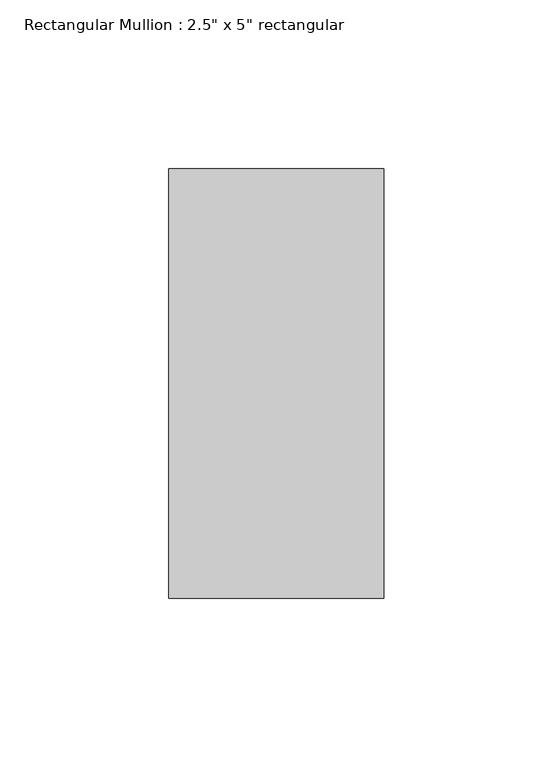
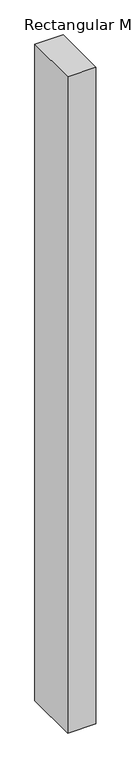
"""IFC4 building model written with IfcOpenShell, lengths in millimetres: member geometry."""

from ifc_helpers import new_model, si_unit, frame, origin, place, context, project, spatial, polyline, outline, extrude, source, transform, mapped, element, save


def member_00c01c4d(model_context):
    return source(origin(), model_context, "Body", "SweptSolid", [
        extrude(outline(polyline([(0.0, 63.5), (0.0, -63.5), (-63.5, -63.5), (-63.5, 63.5), (0.0, 63.5)])), frame((0.0, 0.0, -1555.75), z_axis=(0.0, 0.0, 1.0), x_axis=(1.0, 0.0, 0.0)), (0.0, 0.0, 1.0), 1555.75),
    ])


if __name__ == "__main__":
    model = new_model("IFC4")
    model_context = context("Model", 3, world=origin())
    ifc_project = project(units=[si_unit("LENGTHUNIT", "METRE", prefix="MILLI")], contexts=[model_context])
    site = spatial("IfcSite", under=ifc_project)
    building = spatial("IfcBuilding", under=site)
    placement = place(None, origin())
    member_shape = member_00c01c4d(model_context)
    element("IfcMember", 1, ObjectType="Rectangular Mullion : 2.5\" x 5\" rectangular", at=placement, inside=building, context=model_context, shape_type="MappedRepresentation", body=[
        mapped(member_shape, transform((0.0, 0.0, 0.0), x_axis=(1.0, 0.0, 0.0), y_axis=(0.0, 1.0, 0.0), z_axis=(0.0, 0.0, 1.0))),
    ])
    save(model, "model.ifc")

# Revit data of these elements
# Type "Rectangular Mullion : 2.5\" x 5\" rectangular"
#   built-in parameter 1007304 = 0.416667 (stored number, unit not read)
#   built-in parameter 1007301 = 0.104167 (stored number, unit not read)
#   built-in parameter 1007300 = 0.104167 (stored number, unit not read)
# Element 1 (IfcMember, "Rectangular Mullion : 2.5\" x 5\" rectangular")
#   Materials on its faces: "Aluminum"
# Materials
#   "Aluminum": class "Metal", colour RGB 247 247 247, transparency 0, Description = "Aluminum 6061", Cost = 0
